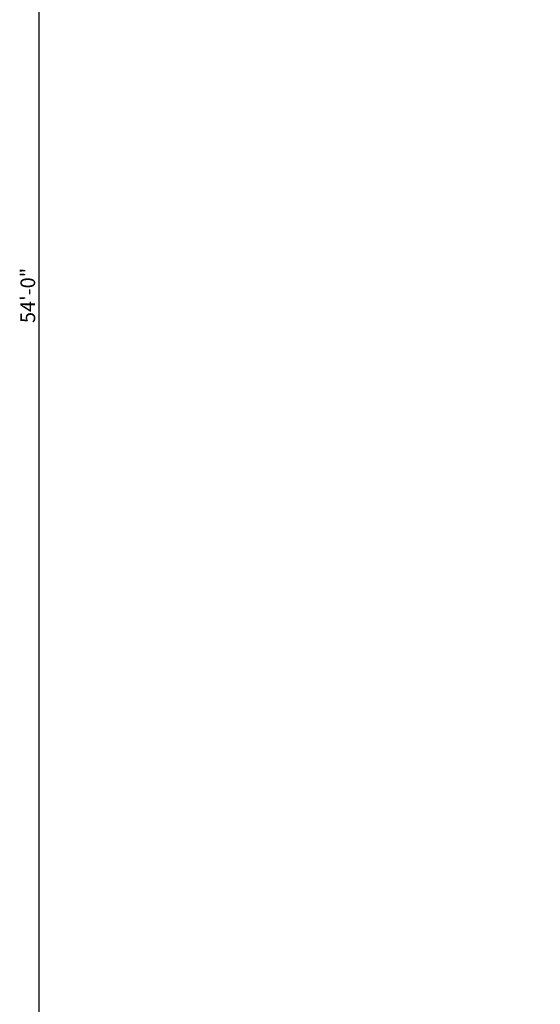
# Model space of a CAD drawing. Units: inches. Extents: x 3283068 to 3284536, y 3240756 to 3241803.
# Tile 2 of 19: x 3283068 to 3283246, y 3241165 to 3241501. Entities that reach past the tile are written whole.
import ezdxf

# ---------------------------------------------------------------- set-up
doc = ezdxf.new("R2010")
doc.units = ezdxf.units.IN
doc.layers.add('A-ANNO-DIMS', color=2, linetype='Continuous', lineweight=18)
doc.styles.get("Standard").update_dxf_attribs({"font": 'arial.ttf'})
doc.dimstyles.new('ISO-25', dxfattribs={"dimtxt": 5, "dimasz": 2.5, "dimexe": 1.25, "dimexo": 0.625, "dimtad": 1, "dimlunit": 4, "dimtxsty": 'Standard', "dimblk": 'ARCHTICK', "dimcen": 2.5, "dimadec": 0, "dimazin": 0, "dimtfac": 1, "dimtmove": 0, "dimatfit": 3, "dimfxl": 1, "dimarcsym": 0})

# ---------------------------------------------------------------- blocks, each defined once
blk = doc.blocks.new('_ArchTick')
at = {"color": 0, "linetype": 'ByBlock', "const_width": 0.15}
blk.add_lwpolyline([(-0.5, -0.5), (0.5, 0.5)], dxfattribs=at)
blk = doc.blocks.new('*D61')
at = {"layer": 'A-ANNO-DIMS', "color": 0, "lineweight": -2, "transparency": 16777216}
for p, q in [((3283247.46, 3241730.6), (3283073.57, 3241730.6)), ((3283074.82, 3241082.6), (3283074.82, 3241730.6)), ((3283247.46, 3241082.6), (3283073.57, 3241082.6))]:
    blk.add_line(p, q, dxfattribs=at)
at = {"layer": 'Defpoints', "color": 0, "transparency": 16777216}
for p in [(3283074.82, 3241730.6), (3283248.09, 3241730.6), (3283248.09, 3241082.6)]:
    blk.add_point(p, dxfattribs=at)
at = {"layer": 'A-ANNO-DIMS', "color": 0, "lineweight": -2, "transparency": 16777216, "xscale": 2.5, "yscale": 2.5, "zscale": 2.5}
for p, rotation in [((3283074.82, 3241730.6), 90), ((3283074.82, 3241082.6), 270)]:
    blk.add_blockref('_ArchTick', p, dxfattribs=dict(at, rotation=rotation))
at = {"layer": 'A-ANNO-DIMS', "color": 0, "transparency": 16777216, "insert": (3283071.64, 3241406.6), "char_height": 5, "attachment_point": 5, "rotation": 90}
blk.add_mtext('54\'-0"', dxfattribs=at)

msp = doc.modelspace()

# ---------------------------------------------------------------- dimensions: what is measured, and where the dimension line sits
at = {"layer": 'A-ANNO-DIMS'}
dim = msp.add_linear_dim(base=(3283074.817, 3241730.602), p1=(3283248.089, 3241082.602), p2=(3283248.089, 3241730.602), angle=90, dimstyle='ISO-25', override={"dimdec": 1, "dimlfac": 1, "dimrnd": 0, "dimzin": 1, "dimdsep": 46, "dimlunit": 4, "dimfrac": 2}, dxfattribs=at)
dim.commit()
dim.dimension.update_dxf_attribs({"geometry": '*D61', "text_midpoint": (3283071.639, 3241406.602)})

doc.saveas('drawing.dxf')
